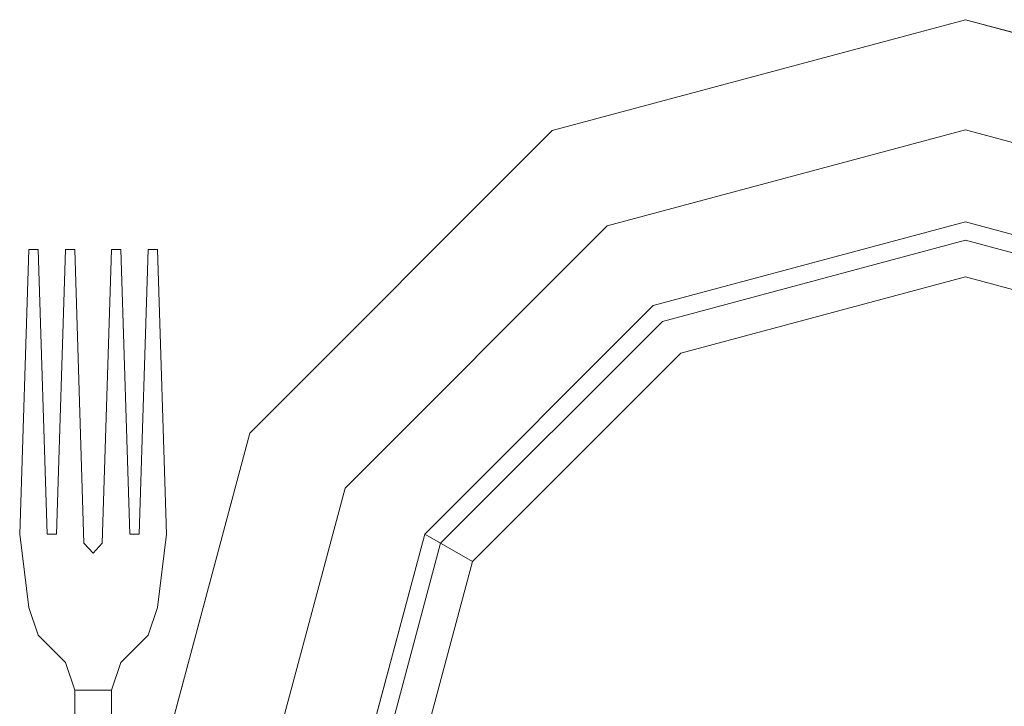
# Model space of a CAD drawing. Units: inches. Extents: x 375 to 1122, y 27 to 1069.
# Tile 11 of 155: x 719.34 to 725.941, y 262.679 to 267.28. Entities that reach past the tile are written whole.
import ezdxf

# ---------------------------------------------------------------- set-up
doc = ezdxf.new("R2010")
doc.units = ezdxf.units.IN
doc.layers.add('Furniture', color=30, linetype='Continuous', lineweight=18)

# ---------------------------------------------------------------- blocks, each defined once
blk = doc.blocks.new('A$C403C54AD')
for p, q in [((2.0741, 0.86135, -0.05014), (2.07871, 0.86289, -0.04968)), ((2.0741, 0.86135, -0.05322), (2.07871, 0.86289, -0.05276))]:
    blk.add_line(p, q)
at = {"linetype": 'ByBlock'}
for points, invisible_edges in [([(2.11411, 1.11993, -0.04398), (2.11411, 1.01834, -0.04398), (2.11411, 1.01834, -0.04398), (2.06332, 1.10632, -0.04398)], 5), ([(2.06332, 1.10632, -0.04398), (2.11411, 1.01834, -0.04398), (2.11411, 1.01834, -0.04398), (2.02614, 1.06914, -0.04398)], 5), ([(1.99415, 1.08761, -0.03783), (2.01014, 1.07837, -0.03783), (1.99406, 1.01834, -0.03783), (1.97559, 1.01834, -0.03783)], 5), ([(2.02347, 1.07068, -0.05168), (1.99415, 1.08761, -0.04244), (1.97559, 1.01834, -0.04244), (2.00945, 1.01834, -0.05168)], 5), ([(2.01014, 1.07837, -0.03783), (2.02614, 1.06914, -0.04398), (2.01253, 1.01834, -0.04398), (1.99406, 1.01834, -0.03783)], 5), ([(2.03147, 1.06606, -0.06091), (2.02347, 1.07068, -0.05168), (2.00945, 1.01834, -0.05168), (2.01868, 1.01834, -0.06091)], 5), ([(2.02614, 1.06914, -0.04398), (2.11411, 1.01834, -0.04398), (2.11411, 1.01834, -0.04398), (2.01253, 1.01834, -0.04398)], 5), ([(1.97559, 1.01834, -0.03783), (1.99406, 1.01834, -0.03783), (2.01014, 0.95832, -0.03783), (1.99415, 0.94908, -0.03783)], 5), ([(2.00945, 1.01834, -0.05168), (1.97559, 1.01834, -0.04244), (1.99415, 0.94908, -0.04244), (2.02347, 0.96601, -0.05168)], 5), ([(1.99406, 1.01834, -0.03783), (2.01253, 1.01834, -0.04398), (2.02614, 0.96755, -0.04398), (2.01014, 0.95832, -0.03783)], 5), ([(2.01868, 1.01834, -0.06091), (2.00945, 1.01834, -0.05168), (2.02347, 0.96601, -0.05168), (2.03147, 0.97063, -0.06091)], 5), ([(2.01253, 1.01834, -0.04398), (2.11411, 1.01834, -0.04398), (2.11411, 1.01834, -0.04398), (2.02614, 0.96755, -0.04398)], 5), ([(2.02614, 0.96755, -0.04398), (2.11411, 1.01834, -0.04398), (2.11411, 1.01834, -0.04398), (2.06332, 0.93037, -0.04398)], 5), ([(2.06332, 0.93037, -0.04398), (2.11411, 1.01834, -0.04398), (2.11411, 1.01834, -0.04398), (2.11411, 0.91676, -0.04398)], 5), ([(2.03147, 0.97063, -0.06091), (2.02347, 0.96601, -0.05168), (2.06178, 0.9277, -0.05168), (2.0664, 0.9357, -0.06091)], 1), ([(2.01014, 0.95832, -0.03783), (2.02614, 0.96755, -0.04398), (2.06332, 0.93037, -0.04398), (2.05409, 0.91437, -0.03783)], 5), ([(2.02347, 0.96601, -0.05168), (1.99415, 0.94908, -0.04244), (2.04485, 0.89838, -0.04244), (2.06178, 0.9277, -0.05168)], 5), ([(1.99415, 0.94908, -0.03783), (2.01014, 0.95832, -0.03783), (2.05409, 0.91437, -0.03783), (2.04485, 0.89838, -0.03783)], 5), ([(2.05409, 0.91437, -0.03783), (2.06332, 0.93037, -0.04398), (2.11411, 0.91676, -0.04398), (2.11411, 0.89829, -0.03783)], 5), ([(2.06178, 0.9277, -0.05168), (2.04485, 0.89838, -0.04244), (2.11411, 0.87982, -0.04244), (2.11411, 0.91368, -0.05168)], 5), ([(2.04485, 0.89838, -0.03783), (2.05409, 0.91437, -0.03783), (2.11411, 0.89829, -0.03783), (2.11411, 0.87982, -0.03783)], 5)]:
    blk.add_3dface(points, dxfattribs=dict(at, invisible_edges=invisible_edges))
for points in [[(1.99415, 1.08761, -0.04244), (1.99415, 1.08761, -0.03783), (1.97559, 1.01834, -0.03783), (1.97559, 1.01834, -0.04244)], [(1.97559, 1.01834, -0.04244), (1.97559, 1.01834, -0.03783), (1.99415, 0.94908, -0.03783), (1.99415, 0.94908, -0.04244)], [(1.99415, 0.94908, -0.04244), (1.99415, 0.94908, -0.03783), (2.04485, 0.89838, -0.03783), (2.04485, 0.89838, -0.04244)], [(2.0664, 0.9357, -0.06091), (2.06178, 0.9277, -0.05168), (2.11411, 0.91368, -0.05168), (2.11411, 0.92291, -0.06091)], [(2.04485, 0.89838, -0.04244), (2.04485, 0.89838, -0.03783), (2.11411, 0.87982, -0.03783), (2.11411, 0.87982, -0.04244)]]:
    blk.add_3dface(points, dxfattribs=at)
for points, invisible_edges in [([(2.06178, 0.87982, -0.04954), (2.06178, 0.88444, -0.04954), (2.01407, 0.8829, -0.04244), (2.01407, 0.88136, -0.04244)], 1), ([(2.06178, 0.87982, -0.05262), (2.06178, 0.88444, -0.05262), (2.01407, 0.8829, -0.04552), (2.01407, 0.88136, -0.04552)], 1), ([(2.0741, 0.8829, -0.05014), (2.06178, 0.87828, -0.04954), (2.06178, 0.87982, -0.04954), (2.06178, 0.88444, -0.04954)], 5), ([(2.0741, 0.8829, -0.05322), (2.06178, 0.87828, -0.05262), (2.06178, 0.87982, -0.05262), (2.06178, 0.88444, -0.05262)], 5), ([(2.0741, 0.8829, -0.05014), (2.0741, 0.8829, -0.05322), (2.06178, 0.88444, -0.05262), (2.06178, 0.88444, -0.04954)], 1), ([(2.0741, 0.8829, -0.05014), (2.06498, 0.87212, -0.04994), (2.06332, 0.87366, -0.04979), (2.06178, 0.87828, -0.04954)], 13), ([(2.0741, 0.8829, -0.05322), (2.06498, 0.87212, -0.05301), (2.06332, 0.87366, -0.05286), (2.06178, 0.87828, -0.05262)], 13), ([(2.0741, 0.8829, -0.05014), (2.06498, 0.87212, -0.04994), (2.0741, 0.86135, -0.05014), (2.0741, 0.8829, -0.05014)], 7), ([(2.0741, 0.8829, -0.05322), (2.06498, 0.87212, -0.05301), (2.0741, 0.86135, -0.05322), (2.0741, 0.8829, -0.05322)], 7), ([(2.07871, 0.88136, -0.04968), (2.07871, 0.86289, -0.04968), (2.0741, 0.86135, -0.05014), (2.0741, 0.8829, -0.05014)], 5), ([(2.07871, 0.88136, -0.05276), (2.07871, 0.86289, -0.05276), (2.0741, 0.86135, -0.05322), (2.0741, 0.8829, -0.05322)], 5), ([(2.07871, 0.88136, -0.05276), (2.07871, 0.88136, -0.04968), (2.0741, 0.8829, -0.05014), (2.0741, 0.8829, -0.05322)], 4), ([(2.08179, 0.86596, -0.05152), (2.08179, 0.87828, -0.05152), (2.07871, 0.88136, -0.05276), (2.07871, 0.86289, -0.05276)], 5), ([(2.08179, 0.86596, -0.04844), (2.08179, 0.87828, -0.04844), (2.07871, 0.88136, -0.04968), (2.07871, 0.86289, -0.04968)], 5), ([(2.06178, 0.87828, -0.04954), (2.06332, 0.87366, -0.04979), (2.01407, 0.8752, -0.04244), (2.01407, 0.87674, -0.04244)], 1), ([(2.06178, 0.87828, -0.05262), (2.06332, 0.87366, -0.05286), (2.01407, 0.8752, -0.04552), (2.01407, 0.87674, -0.04552)], 1), ([(2.08333, 0.8675, -0.04739), (2.08333, 0.87674, -0.04739), (2.08179, 0.87828, -0.04844), (2.08179, 0.86596, -0.04844)], 5), ([(2.08333, 0.8675, -0.05018), (2.08333, 0.87674, -0.05018), (2.08179, 0.87828, -0.05152), (2.08179, 0.86596, -0.05152)], 5), ([(2.08333, 0.87674, -0.05018), (2.08333, 0.87674, -0.04739), (2.08179, 0.87828, -0.04844), (2.08179, 0.87828, -0.05152)], 1), ([(2.08795, 0.8752, -0.04504), (2.08795, 0.86904, -0.04504), (2.08333, 0.8675, -0.04739), (2.08333, 0.87674, -0.04739)], 4), ([(2.08795, 0.8752, -0.04504), (2.08795, 0.8752, -0.04763), (2.08333, 0.87674, -0.05018), (2.08333, 0.87674, -0.04739)], 5), ([(2.08795, 0.8752, -0.04763), (2.08795, 0.86904, -0.04763), (2.08333, 0.8675, -0.05018), (2.08333, 0.87674, -0.05018)], 4), ([(2.09872, 0.8752, -0.04555), (2.09872, 0.8752, -0.04296), (2.08795, 0.8752, -0.04504), (2.08795, 0.8752, -0.04763)], 5), ([(2.0741, 0.86135, -0.05014), (2.06498, 0.87212, -0.04994), (2.06332, 0.87058, -0.04979), (2.06178, 0.86596, -0.04954)], 13), ([(2.0741, 0.86135, -0.05322), (2.06498, 0.87212, -0.05301), (2.06332, 0.87058, -0.05286), (2.06178, 0.86596, -0.05262)], 13), ([(2.06332, 0.87058, -0.04979), (2.06178, 0.86596, -0.04954), (2.01407, 0.8675, -0.04244), (2.01407, 0.86904, -0.04244)], 1), ([(2.06332, 0.87058, -0.05286), (2.06178, 0.86596, -0.05262), (2.01407, 0.8675, -0.04552), (2.01407, 0.86904, -0.04552)], 1), ([(2.08795, 0.86904, -0.04763), (2.08795, 0.86904, -0.04504), (2.08333, 0.8675, -0.04739), (2.08333, 0.8675, -0.05018)], 5), ([(2.08795, 0.86904, -0.04763), (2.08795, 0.86904, -0.04504), (2.09872, 0.86904, -0.04296), (2.09872, 0.86904, -0.04555)], 5), ([(2.08333, 0.8675, -0.04739), (2.08333, 0.8675, -0.05018), (2.08179, 0.86596, -0.05152), (2.08179, 0.86596, -0.04844)], 1), ([(2.0741, 0.86135, -0.05014), (2.06178, 0.86596, -0.04954), (2.06178, 0.86443, -0.04954), (2.06178, 0.85981, -0.04954)], 5), ([(2.0741, 0.86135, -0.05322), (2.06178, 0.86596, -0.05262), (2.06178, 0.86443, -0.05262), (2.06178, 0.85981, -0.05262)], 5), ([(2.06178, 0.86443, -0.04954), (2.06178, 0.85981, -0.04954), (2.01407, 0.86135, -0.04244), (2.01407, 0.86289, -0.04244)], 1), ([(2.06178, 0.86443, -0.05262), (2.06178, 0.85981, -0.05262), (2.01407, 0.86135, -0.04552), (2.01407, 0.86289, -0.04552)], 1), ([(2.07871, 0.86289, -0.04968), (2.07871, 0.86289, -0.05276), (2.0741, 0.86135, -0.05322), (2.0741, 0.86135, -0.05014)], 4), ([(2.0741, 0.86135, -0.05322), (2.0741, 0.86135, -0.05014), (2.06178, 0.85981, -0.04954), (2.06178, 0.85981, -0.05262)], 1)]:
    blk.add_3dface(points, dxfattribs=dict(invisible_edges=invisible_edges))
for points in [[(2.06178, 0.88444, -0.05262), (2.06178, 0.88444, -0.04954), (2.01407, 0.8829, -0.04244), (2.01407, 0.8829, -0.04552)], [(2.01407, 0.8829, -0.04552), (2.01407, 0.8829, -0.04244), (2.01407, 0.88136, -0.04244), (2.01407, 0.88136, -0.04552)], [(2.01407, 0.88136, -0.04244), (2.01407, 0.88136, -0.04552), (2.06178, 0.87982, -0.05262), (2.06178, 0.87982, -0.04954)], [(2.06178, 0.87828, -0.05262), (2.06178, 0.87828, -0.04954), (2.06178, 0.87982, -0.04954), (2.06178, 0.87982, -0.05262)], [(2.08179, 0.87828, -0.04844), (2.08179, 0.87828, -0.05152), (2.07871, 0.88136, -0.05276), (2.07871, 0.88136, -0.04968)], [(2.06178, 0.87828, -0.05262), (2.06178, 0.87828, -0.04954), (2.01407, 0.87674, -0.04244), (2.01407, 0.87674, -0.04552)], [(2.01407, 0.87674, -0.04552), (2.01407, 0.87674, -0.04244), (2.01407, 0.8752, -0.04244), (2.01407, 0.8752, -0.04552)], [(2.01407, 0.8752, -0.04552), (2.01407, 0.8752, -0.04244), (2.06332, 0.87366, -0.04979), (2.06332, 0.87366, -0.05286)], [(2.09872, 0.86904, -0.04296), (2.09872, 0.8752, -0.04296), (2.08795, 0.8752, -0.04504), (2.08795, 0.86904, -0.04504)], [(2.09872, 0.86904, -0.04555), (2.09872, 0.8752, -0.04555), (2.08795, 0.8752, -0.04763), (2.08795, 0.86904, -0.04763)], [(2.06498, 0.87212, -0.05301), (2.06498, 0.87212, -0.04994), (2.06332, 0.87366, -0.04979), (2.06332, 0.87366, -0.05286)], [(2.06332, 0.87058, -0.04979), (2.06332, 0.87058, -0.05286), (2.06498, 0.87212, -0.05301), (2.06498, 0.87212, -0.04994)], [(2.06332, 0.87058, -0.05286), (2.06332, 0.87058, -0.04979), (2.01407, 0.86904, -0.04244), (2.01407, 0.86904, -0.04552)], [(2.01407, 0.86904, -0.04552), (2.01407, 0.86904, -0.04244), (2.01407, 0.8675, -0.04244), (2.01407, 0.8675, -0.04552)], [(2.01407, 0.8675, -0.04244), (2.01407, 0.8675, -0.04552), (2.06178, 0.86596, -0.05262), (2.06178, 0.86596, -0.04954)], [(2.06178, 0.86443, -0.04954), (2.06178, 0.86443, -0.05262), (2.06178, 0.86596, -0.05262), (2.06178, 0.86596, -0.04954)], [(2.08179, 0.86596, -0.05152), (2.08179, 0.86596, -0.04844), (2.07871, 0.86289, -0.04968), (2.07871, 0.86289, -0.05276)], [(2.06178, 0.86443, -0.04954), (2.06178, 0.86443, -0.05262), (2.01407, 0.86289, -0.04552), (2.01407, 0.86289, -0.04244)], [(2.01407, 0.86289, -0.04552), (2.01407, 0.86289, -0.04244), (2.01407, 0.86135, -0.04244), (2.01407, 0.86135, -0.04552)], [(2.01407, 0.86135, -0.04244), (2.01407, 0.86135, -0.04552), (2.06178, 0.85981, -0.05262), (2.06178, 0.85981, -0.04954)]]:
    blk.add_3dface(points)

msp = doc.modelspace()

# ---------------------------------------------------------------- block references
at = {"layer": 'Furniture', "xscale": 39.9918517141215, "yscale": 39.9918517141215, "zscale": 39.9918517141215, "rotation": 270}
msp.add_blockref('A$C403C54AD', (684.9549, 346.2875, 0.024), dxfattribs=at)

doc.saveas('drawing.dxf')
